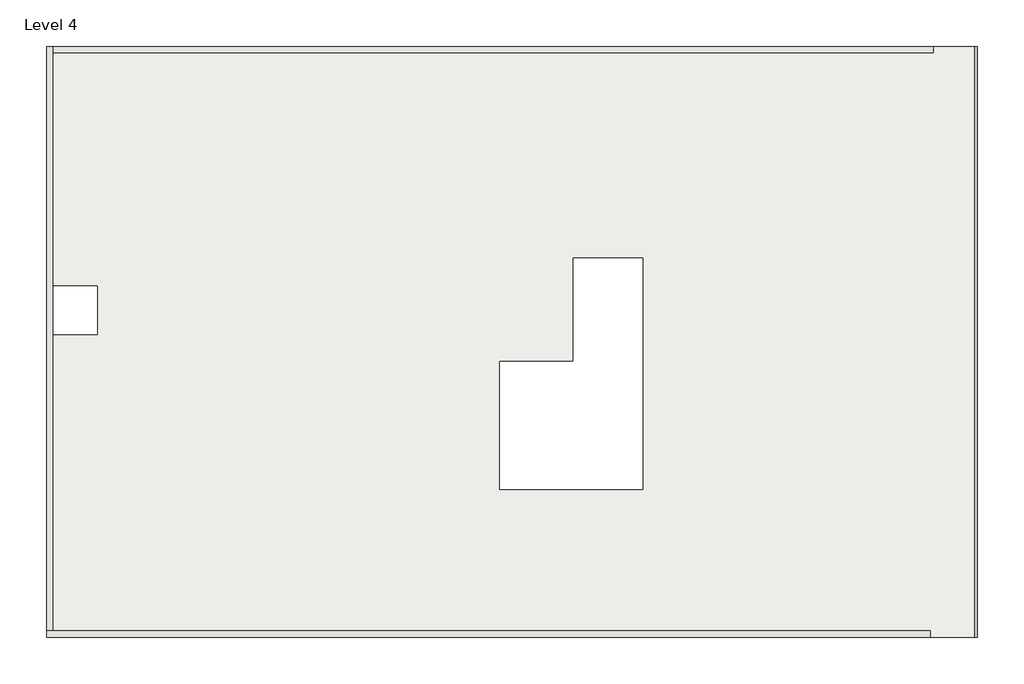
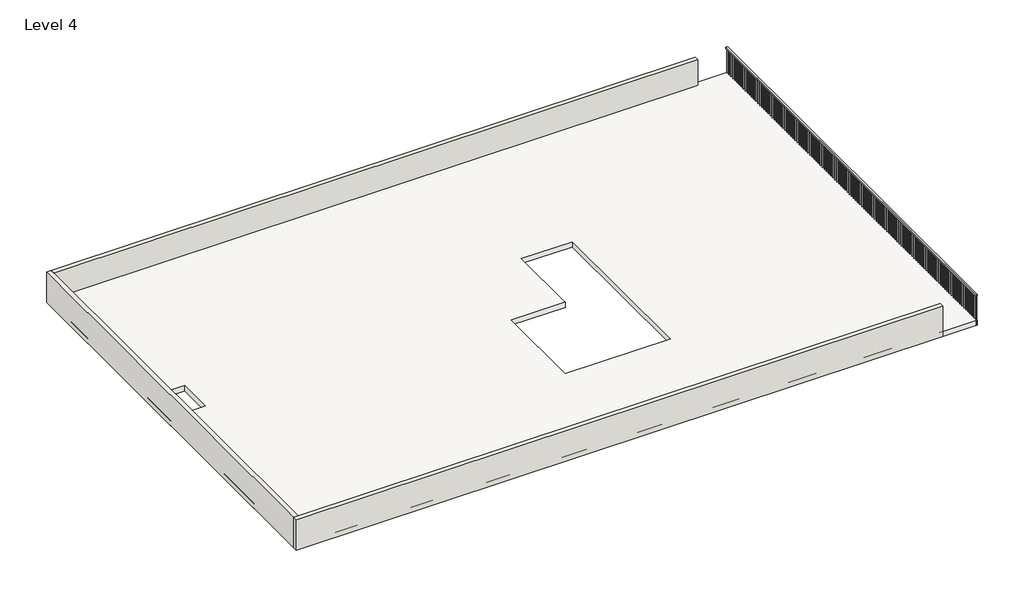
# One storey: 3 walls, 1 railing, 1 slab.
"""IFC4 building model written with IfcOpenShell, lengths in millimetres."""

from ifc_helpers import new_model, si_unit, frame, origin, place, context, project, spatial, polyline, outline, extrude, faceted_brep, element, save

model = new_model("IFC4")

# Units and contexts
model_context = context("Model", 3, world=origin())
ifc_project = project(units=[si_unit("LENGTHUNIT", "METRE", prefix="MILLI")], contexts=[model_context])

# Site, building, storey
site = spatial("IfcSite", under=ifc_project)
building = spatial("IfcBuilding", under=site)
storey = spatial("IfcBuildingStorey", under=building, Name="Level 4", Elevation=9144.0)

# Railing
placement = place(None, origin())
element("IfcRailing", 1, ObjectType="Handrail - Rectangular", at=placement, inside=storey, context=model_context, shape_type="SweptSolid", body=[
    extrude(outline(polyline([(6706.5574466, 3231.2168492), (6757.3574466, 3231.2168492), (6757.3574466, -8960.7831508), (6706.5574466, -8960.7831508), (6706.5574466, 3231.2168492)])), frame((0.0, 0.0, 10007.6), z_axis=(0.0, 0.0, 1.0), x_axis=(1.0, 0.0, 0.0)), (0.0, 0.0, 1.0), 50.8),
    extrude(outline(polyline([(6722.4324466, -8849.6581508), (6741.4824466, -8849.6581508), (6741.4824466, -8868.7081508), (6722.4324466, -8868.7081508), (6722.4324466, -8849.6581508)])), frame((0.0, 0.0, 9144.0), z_axis=(0.0, 0.0, 1.0), x_axis=(1.0, 0.0, 0.0)), (0.0, 0.0, 1.0), 863.6),
    extrude(outline(polyline([(6722.4324466, -8748.0581508), (6741.4824466, -8748.0581508), (6741.4824466, -8767.1081508), (6722.4324466, -8767.1081508), (6722.4324466, -8748.0581508)])), frame((0.0, 0.0, 9144.0), z_axis=(0.0, 0.0, 1.0), x_axis=(1.0, 0.0, 0.0)), (0.0, 0.0, 1.0), 863.6),
    extrude(outline(polyline([(6722.4324466, -8646.4581508), (6741.4824466, -8646.4581508), (6741.4824466, -8665.5081508), (6722.4324466, -8665.5081508), (6722.4324466, -8646.4581508)])), frame((0.0, 0.0, 9144.0), z_axis=(0.0, 0.0, 1.0), x_axis=(1.0, 0.0, 0.0)), (0.0, 0.0, 1.0), 863.6),
    extrude(outline(polyline([(6722.4324466, -8544.8581508), (6741.4824466, -8544.8581508), (6741.4824466, -8563.9081508), (6722.4324466, -8563.9081508), (6722.4324466, -8544.8581508)])), frame((0.0, 0.0, 9144.0), z_axis=(0.0, 0.0, 1.0), x_axis=(1.0, 0.0, 0.0)), (0.0, 0.0, 1.0), 863.6),
    extrude(outline(polyline([(6722.4324466, -8443.2581508), (6741.4824466, -8443.2581508), (6741.4824466, -8462.3081508), (6722.4324466, -8462.3081508), (6722.4324466, -8443.2581508)])), frame((0.0, 0.0, 9144.0), z_axis=(0.0, 0.0, 1.0), x_axis=(1.0, 0.0, 0.0)), (0.0, 0.0, 1.0), 863.6),
    extrude(outline(polyline([(6722.4324466, -8341.6581508), (6741.4824466, -8341.6581508), (6741.4824466, -8360.7081508), (6722.4324466, -8360.7081508), (6722.4324466, -8341.6581508)])), frame((0.0, 0.0, 9144.0), z_axis=(0.0, 0.0, 1.0), x_axis=(1.0, 0.0, 0.0)), (0.0, 0.0, 1.0), 863.6),
    extrude(outline(polyline([(6722.4324466, -8240.0581508), (6741.4824466, -8240.0581508), (6741.4824466, -8259.1081508), (6722.4324466, -8259.1081508), (6722.4324466, -8240.0581508)])), frame((0.0, 0.0, 9144.0), z_axis=(0.0, 0.0, 1.0), x_axis=(1.0, 0.0, 0.0)), (0.0, 0.0, 1.0), 863.6),
    extrude(outline(polyline([(6722.4324466, -8138.4581508), (6741.4824466, -8138.4581508), (6741.4824466, -8157.5081508), (6722.4324466, -8157.5081508), (6722.4324466, -8138.4581508)])), frame((0.0, 0.0, 9144.0), z_axis=(0.0, 0.0, 1.0), x_axis=(1.0, 0.0, 0.0)), (0.0, 0.0, 1.0), 863.6),
    extrude(outline(polyline([(6722.4324466, -8036.8581508), (6741.4824466, -8036.8581508), (6741.4824466, -8055.9081508), (6722.4324466, -8055.9081508), (6722.4324466, -8036.8581508)])), frame((0.0, 0.0, 9144.0), z_axis=(0.0, 0.0, 1.0), x_axis=(1.0, 0.0, 0.0)), (0.0, 0.0, 1.0), 863.6),
    extrude(outline(polyline([(6722.4324466, -7935.2581508), (6741.4824466, -7935.2581508), (6741.4824466, -7954.3081508), (6722.4324466, -7954.3081508), (6722.4324466, -7935.2581508)])), frame((0.0, 0.0, 9144.0), z_axis=(0.0, 0.0, 1.0), x_axis=(1.0, 0.0, 0.0)), (0.0, 0.0, 1.0), 863.6),
    extrude(outline(polyline([(6722.4324466, -7833.6581508), (6741.4824466, -7833.6581508), (6741.4824466, -7852.7081508), (6722.4324466, -7852.7081508), (6722.4324466, -7833.6581508)])), frame((0.0, 0.0, 9144.0), z_axis=(0.0, 0.0, 1.0), x_axis=(1.0, 0.0, 0.0)), (0.0, 0.0, 1.0), 863.6),
    extrude(outline(polyline([(6722.4324466, -7732.0581508), (6741.4824466, -7732.0581508), (6741.4824466, -7751.1081508), (6722.4324466, -7751.1081508), (6722.4324466, -7732.0581508)])), frame((0.0, 0.0, 9144.0), z_axis=(0.0, 0.0, 1.0), x_axis=(1.0, 0.0, 0.0)), (0.0, 0.0, 1.0), 863.6),
    extrude(outline(polyline([(6722.4324466, -7630.4581508), (6741.4824466, -7630.4581508), (6741.4824466, -7649.5081508), (6722.4324466, -7649.5081508), (6722.4324466, -7630.4581508)])), frame((0.0, 0.0, 9144.0), z_axis=(0.0, 0.0, 1.0), x_axis=(1.0, 0.0, 0.0)), (0.0, 0.0, 1.0), 863.6),
    extrude(outline(polyline([(6722.4324466, -7528.8581508), (6741.4824466, -7528.8581508), (6741.4824466, -7547.9081508), (6722.4324466, -7547.9081508), (6722.4324466, -7528.8581508)])), frame((0.0, 0.0, 9144.0), z_axis=(0.0, 0.0, 1.0), x_axis=(1.0, 0.0, 0.0)), (0.0, 0.0, 1.0), 863.6),
    extrude(outline(polyline([(6722.4324466, -7427.2581508), (6741.4824466, -7427.2581508), (6741.4824466, -7446.3081508), (6722.4324466, -7446.3081508), (6722.4324466, -7427.2581508)])), frame((0.0, 0.0, 9144.0), z_axis=(0.0, 0.0, 1.0), x_axis=(1.0, 0.0, 0.0)), (0.0, 0.0, 1.0), 863.6),
    extrude(outline(polyline([(6722.4324466, -7325.6581508), (6741.4824466, -7325.6581508), (6741.4824466, -7344.7081508), (6722.4324466, -7344.7081508), (6722.4324466, -7325.6581508)])), frame((0.0, 0.0, 9144.0), z_axis=(0.0, 0.0, 1.0), x_axis=(1.0, 0.0, 0.0)), (0.0, 0.0, 1.0), 863.6),
    extrude(outline(polyline([(6722.4324466, -7224.0581508), (6741.4824466, -7224.0581508), (6741.4824466, -7243.1081508), (6722.4324466, -7243.1081508), (6722.4324466, -7224.0581508)])), frame((0.0, 0.0, 9144.0), z_axis=(0.0, 0.0, 1.0), x_axis=(1.0, 0.0, 0.0)), (0.0, 0.0, 1.0), 863.6),
    extrude(outline(polyline([(6722.4324466, -7122.4581508), (6741.4824466, -7122.4581508), (6741.4824466, -7141.5081508), (6722.4324466, -7141.5081508), (6722.4324466, -7122.4581508)])), frame((0.0, 0.0, 9144.0), z_axis=(0.0, 0.0, 1.0), x_axis=(1.0, 0.0, 0.0)), (0.0, 0.0, 1.0), 863.6),
    extrude(outline(polyline([(6722.4324466, -7020.8581508), (6741.4824466, -7020.8581508), (6741.4824466, -7039.9081508), (6722.4324466, -7039.9081508), (6722.4324466, -7020.8581508)])), frame((0.0, 0.0, 9144.0), z_axis=(0.0, 0.0, 1.0), x_axis=(1.0, 0.0, 0.0)), (0.0, 0.0, 1.0), 863.6),
    extrude(outline(polyline([(6722.4324466, -6919.2581508), (6741.4824466, -6919.2581508), (6741.4824466, -6938.3081508), (6722.4324466, -6938.3081508), (6722.4324466, -6919.2581508)])), frame((0.0, 0.0, 9144.0), z_axis=(0.0, 0.0, 1.0), x_axis=(1.0, 0.0, 0.0)), (0.0, 0.0, 1.0), 863.6),
    extrude(outline(polyline([(6722.4324466, -6817.6581508), (6741.4824466, -6817.6581508), (6741.4824466, -6836.7081508), (6722.4324466, -6836.7081508), (6722.4324466, -6817.6581508)])), frame((0.0, 0.0, 9144.0), z_axis=(0.0, 0.0, 1.0), x_axis=(1.0, 0.0, 0.0)), (0.0, 0.0, 1.0), 863.6),
    extrude(outline(polyline([(6722.4324466, -6716.0581508), (6741.4824466, -6716.0581508), (6741.4824466, -6735.1081508), (6722.4324466, -6735.1081508), (6722.4324466, -6716.0581508)])), frame((0.0, 0.0, 9144.0), z_axis=(0.0, 0.0, 1.0), x_axis=(1.0, 0.0, 0.0)), (0.0, 0.0, 1.0), 863.6),
    extrude(outline(polyline([(6722.4324466, -6614.4581508), (6741.4824466, -6614.4581508), (6741.4824466, -6633.5081508), (6722.4324466, -6633.5081508), (6722.4324466, -6614.4581508)])), frame((0.0, 0.0, 9144.0), z_axis=(0.0, 0.0, 1.0), x_axis=(1.0, 0.0, 0.0)), (0.0, 0.0, 1.0), 863.6),
    extrude(outline(polyline([(6722.4324466, -6512.8581508), (6741.4824466, -6512.8581508), (6741.4824466, -6531.9081508), (6722.4324466, -6531.9081508), (6722.4324466, -6512.8581508)])), frame((0.0, 0.0, 9144.0), z_axis=(0.0, 0.0, 1.0), x_axis=(1.0, 0.0, 0.0)), (0.0, 0.0, 1.0), 863.6),
    extrude(outline(polyline([(6722.4324466, -6411.2581508), (6741.4824466, -6411.2581508), (6741.4824466, -6430.3081508), (6722.4324466, -6430.3081508), (6722.4324466, -6411.2581508)])), frame((0.0, 0.0, 9144.0), z_axis=(0.0, 0.0, 1.0), x_axis=(1.0, 0.0, 0.0)), (0.0, 0.0, 1.0), 863.6),
    extrude(outline(polyline([(6722.4324466, -6309.6581508), (6741.4824466, -6309.6581508), (6741.4824466, -6328.7081508), (6722.4324466, -6328.7081508), (6722.4324466, -6309.6581508)])), frame((0.0, 0.0, 9144.0), z_axis=(0.0, 0.0, 1.0), x_axis=(1.0, 0.0, 0.0)), (0.0, 0.0, 1.0), 863.6),
    extrude(outline(polyline([(6722.4324466, -6208.0581508), (6741.4824466, -6208.0581508), (6741.4824466, -6227.1081508), (6722.4324466, -6227.1081508), (6722.4324466, -6208.0581508)])), frame((0.0, 0.0, 9144.0), z_axis=(0.0, 0.0, 1.0), x_axis=(1.0, 0.0, 0.0)), (0.0, 0.0, 1.0), 863.6),
    extrude(outline(polyline([(6722.4324466, -6106.4581508), (6741.4824466, -6106.4581508), (6741.4824466, -6125.5081508), (6722.4324466, -6125.5081508), (6722.4324466, -6106.4581508)])), frame((0.0, 0.0, 9144.0), z_axis=(0.0, 0.0, 1.0), x_axis=(1.0, 0.0, 0.0)), (0.0, 0.0, 1.0), 863.6),
    extrude(outline(polyline([(6722.4324466, -6004.8581508), (6741.4824466, -6004.8581508), (6741.4824466, -6023.9081508), (6722.4324466, -6023.9081508), (6722.4324466, -6004.8581508)])), frame((0.0, 0.0, 9144.0), z_axis=(0.0, 0.0, 1.0), x_axis=(1.0, 0.0, 0.0)), (0.0, 0.0, 1.0), 863.6),
    extrude(outline(polyline([(6722.4324466, -5903.2581508), (6741.4824466, -5903.2581508), (6741.4824466, -5922.3081508), (6722.4324466, -5922.3081508), (6722.4324466, -5903.2581508)])), frame((0.0, 0.0, 9144.0), z_axis=(0.0, 0.0, 1.0), x_axis=(1.0, 0.0, 0.0)), (0.0, 0.0, 1.0), 863.6),
    extrude(outline(polyline([(6722.4324466, -5801.6581508), (6741.4824466, -5801.6581508), (6741.4824466, -5820.7081508), (6722.4324466, -5820.7081508), (6722.4324466, -5801.6581508)])), frame((0.0, 0.0, 9144.0), z_axis=(0.0, 0.0, 1.0), x_axis=(1.0, 0.0, 0.0)), (0.0, 0.0, 1.0), 863.6),
    extrude(outline(polyline([(6722.4324466, -5700.0581508), (6741.4824466, -5700.0581508), (6741.4824466, -5719.1081508), (6722.4324466, -5719.1081508), (6722.4324466, -5700.0581508)])), frame((0.0, 0.0, 9144.0), z_axis=(0.0, 0.0, 1.0), x_axis=(1.0, 0.0, 0.0)), (0.0, 0.0, 1.0), 863.6),
    extrude(outline(polyline([(6722.4324466, -5598.4581508), (6741.4824466, -5598.4581508), (6741.4824466, -5617.5081508), (6722.4324466, -5617.5081508), (6722.4324466, -5598.4581508)])), frame((0.0, 0.0, 9144.0), z_axis=(0.0, 0.0, 1.0), x_axis=(1.0, 0.0, 0.0)), (0.0, 0.0, 1.0), 863.6),
    extrude(outline(polyline([(6722.4324466, -5496.8581508), (6741.4824466, -5496.8581508), (6741.4824466, -5515.9081508), (6722.4324466, -5515.9081508), (6722.4324466, -5496.8581508)])), frame((0.0, 0.0, 9144.0), z_axis=(0.0, 0.0, 1.0), x_axis=(1.0, 0.0, 0.0)), (0.0, 0.0, 1.0), 863.6),
    extrude(outline(polyline([(6722.4324466, -5395.2581508), (6741.4824466, -5395.2581508), (6741.4824466, -5414.3081508), (6722.4324466, -5414.3081508), (6722.4324466, -5395.2581508)])), frame((0.0, 0.0, 9144.0), z_axis=(0.0, 0.0, 1.0), x_axis=(1.0, 0.0, 0.0)), (0.0, 0.0, 1.0), 863.6),
    extrude(outline(polyline([(6722.4324466, -5293.6581508), (6741.4824466, -5293.6581508), (6741.4824466, -5312.7081508), (6722.4324466, -5312.7081508), (6722.4324466, -5293.6581508)])), frame((0.0, 0.0, 9144.0), z_axis=(0.0, 0.0, 1.0), x_axis=(1.0, 0.0, 0.0)), (0.0, 0.0, 1.0), 863.6),
    extrude(outline(polyline([(6722.4324466, -5192.0581508), (6741.4824466, -5192.0581508), (6741.4824466, -5211.1081508), (6722.4324466, -5211.1081508), (6722.4324466, -5192.0581508)])), frame((0.0, 0.0, 9144.0), z_axis=(0.0, 0.0, 1.0), x_axis=(1.0, 0.0, 0.0)), (0.0, 0.0, 1.0), 863.6),
    extrude(outline(polyline([(6722.4324466, -5090.4581508), (6741.4824466, -5090.4581508), (6741.4824466, -5109.5081508), (6722.4324466, -5109.5081508), (6722.4324466, -5090.4581508)])), frame((0.0, 0.0, 9144.0), z_axis=(0.0, 0.0, 1.0), x_axis=(1.0, 0.0, 0.0)), (0.0, 0.0, 1.0), 863.6),
    extrude(outline(polyline([(6722.4324466, -4988.8581508), (6741.4824466, -4988.8581508), (6741.4824466, -5007.9081508), (6722.4324466, -5007.9081508), (6722.4324466, -4988.8581508)])), frame((0.0, 0.0, 9144.0), z_axis=(0.0, 0.0, 1.0), x_axis=(1.0, 0.0, 0.0)), (0.0, 0.0, 1.0), 863.6),
    extrude(outline(polyline([(6722.4324466, -4887.2581508), (6741.4824466, -4887.2581508), (6741.4824466, -4906.3081508), (6722.4324466, -4906.3081508), (6722.4324466, -4887.2581508)])), frame((0.0, 0.0, 9144.0), z_axis=(0.0, 0.0, 1.0), x_axis=(1.0, 0.0, 0.0)), (0.0, 0.0, 1.0), 863.6),
    extrude(outline(polyline([(6722.4324466, -4785.6581508), (6741.4824466, -4785.6581508), (6741.4824466, -4804.7081508), (6722.4324466, -4804.7081508), (6722.4324466, -4785.6581508)])), frame((0.0, 0.0, 9144.0), z_axis=(0.0, 0.0, 1.0), x_axis=(1.0, 0.0, 0.0)), (0.0, 0.0, 1.0), 863.6),
    extrude(outline(polyline([(6722.4324466, -4684.0581508), (6741.4824466, -4684.0581508), (6741.4824466, -4703.1081508), (6722.4324466, -4703.1081508), (6722.4324466, -4684.0581508)])), frame((0.0, 0.0, 9144.0), z_axis=(0.0, 0.0, 1.0), x_axis=(1.0, 0.0, 0.0)), (0.0, 0.0, 1.0), 863.6),
    extrude(outline(polyline([(6722.4324466, -4582.4581508), (6741.4824466, -4582.4581508), (6741.4824466, -4601.5081508), (6722.4324466, -4601.5081508), (6722.4324466, -4582.4581508)])), frame((0.0, 0.0, 9144.0), z_axis=(0.0, 0.0, 1.0), x_axis=(1.0, 0.0, 0.0)), (0.0, 0.0, 1.0), 863.6),
    extrude(outline(polyline([(6722.4324466, -4480.8581508), (6741.4824466, -4480.8581508), (6741.4824466, -4499.9081508), (6722.4324466, -4499.9081508), (6722.4324466, -4480.8581508)])), frame((0.0, 0.0, 9144.0), z_axis=(0.0, 0.0, 1.0), x_axis=(1.0, 0.0, 0.0)), (0.0, 0.0, 1.0), 863.6),
    extrude(outline(polyline([(6722.4324466, -4379.2581508), (6741.4824466, -4379.2581508), (6741.4824466, -4398.3081508), (6722.4324466, -4398.3081508), (6722.4324466, -4379.2581508)])), frame((0.0, 0.0, 9144.0), z_axis=(0.0, 0.0, 1.0), x_axis=(1.0, 0.0, 0.0)), (0.0, 0.0, 1.0), 863.6),
    extrude(outline(polyline([(6722.4324466, -4277.6581508), (6741.4824466, -4277.6581508), (6741.4824466, -4296.7081508), (6722.4324466, -4296.7081508), (6722.4324466, -4277.6581508)])), frame((0.0, 0.0, 9144.0), z_axis=(0.0, 0.0, 1.0), x_axis=(1.0, 0.0, 0.0)), (0.0, 0.0, 1.0), 863.6),
    extrude(outline(polyline([(6722.4324466, -4176.0581508), (6741.4824466, -4176.0581508), (6741.4824466, -4195.1081508), (6722.4324466, -4195.1081508), (6722.4324466, -4176.0581508)])), frame((0.0, 0.0, 9144.0), z_axis=(0.0, 0.0, 1.0), x_axis=(1.0, 0.0, 0.0)), (0.0, 0.0, 1.0), 863.6),
    extrude(outline(polyline([(6722.4324466, -4074.4581508), (6741.4824466, -4074.4581508), (6741.4824466, -4093.5081508), (6722.4324466, -4093.5081508), (6722.4324466, -4074.4581508)])), frame((0.0, 0.0, 9144.0), z_axis=(0.0, 0.0, 1.0), x_axis=(1.0, 0.0, 0.0)), (0.0, 0.0, 1.0), 863.6),
    extrude(outline(polyline([(6722.4324466, -3972.8581508), (6741.4824466, -3972.8581508), (6741.4824466, -3991.9081508), (6722.4324466, -3991.9081508), (6722.4324466, -3972.8581508)])), frame((0.0, 0.0, 9144.0), z_axis=(0.0, 0.0, 1.0), x_axis=(1.0, 0.0, 0.0)), (0.0, 0.0, 1.0), 863.6),
    extrude(outline(polyline([(6722.4324466, -3871.2581508), (6741.4824466, -3871.2581508), (6741.4824466, -3890.3081508), (6722.4324466, -3890.3081508), (6722.4324466, -3871.2581508)])), frame((0.0, 0.0, 9144.0), z_axis=(0.0, 0.0, 1.0), x_axis=(1.0, 0.0, 0.0)), (0.0, 0.0, 1.0), 863.6),
    extrude(outline(polyline([(6722.4324466, -3769.6581508), (6741.4824466, -3769.6581508), (6741.4824466, -3788.7081508), (6722.4324466, -3788.7081508), (6722.4324466, -3769.6581508)])), frame((0.0, 0.0, 9144.0), z_axis=(0.0, 0.0, 1.0), x_axis=(1.0, 0.0, 0.0)), (0.0, 0.0, 1.0), 863.6),
    extrude(outline(polyline([(6722.4324466, -3668.0581508), (6741.4824466, -3668.0581508), (6741.4824466, -3687.1081508), (6722.4324466, -3687.1081508), (6722.4324466, -3668.0581508)])), frame((0.0, 0.0, 9144.0), z_axis=(0.0, 0.0, 1.0), x_axis=(1.0, 0.0, 0.0)), (0.0, 0.0, 1.0), 863.6),
    extrude(outline(polyline([(6722.4324466, -3566.4581508), (6741.4824466, -3566.4581508), (6741.4824466, -3585.5081508), (6722.4324466, -3585.5081508), (6722.4324466, -3566.4581508)])), frame((0.0, 0.0, 9144.0), z_axis=(0.0, 0.0, 1.0), x_axis=(1.0, 0.0, 0.0)), (0.0, 0.0, 1.0), 863.6),
    extrude(outline(polyline([(6722.4324466, -3464.8581508), (6741.4824466, -3464.8581508), (6741.4824466, -3483.9081508), (6722.4324466, -3483.9081508), (6722.4324466, -3464.8581508)])), frame((0.0, 0.0, 9144.0), z_axis=(0.0, 0.0, 1.0), x_axis=(1.0, 0.0, 0.0)), (0.0, 0.0, 1.0), 863.6),
    extrude(outline(polyline([(6722.4324466, -3363.2581508), (6741.4824466, -3363.2581508), (6741.4824466, -3382.3081508), (6722.4324466, -3382.3081508), (6722.4324466, -3363.2581508)])), frame((0.0, 0.0, 9144.0), z_axis=(0.0, 0.0, 1.0), x_axis=(1.0, 0.0, 0.0)), (0.0, 0.0, 1.0), 863.6),
    extrude(outline(polyline([(6722.4324466, -3261.6581508), (6741.4824466, -3261.6581508), (6741.4824466, -3280.7081508), (6722.4324466, -3280.7081508), (6722.4324466, -3261.6581508)])), frame((0.0, 0.0, 9144.0), z_axis=(0.0, 0.0, 1.0), x_axis=(1.0, 0.0, 0.0)), (0.0, 0.0, 1.0), 863.6),
    extrude(outline(polyline([(6722.4324466, -3160.0581508), (6741.4824466, -3160.0581508), (6741.4824466, -3179.1081508), (6722.4324466, -3179.1081508), (6722.4324466, -3160.0581508)])), frame((0.0, 0.0, 9144.0), z_axis=(0.0, 0.0, 1.0), x_axis=(1.0, 0.0, 0.0)), (0.0, 0.0, 1.0), 863.6),
    extrude(outline(polyline([(6722.4324466, -3058.4581508), (6741.4824466, -3058.4581508), (6741.4824466, -3077.5081508), (6722.4324466, -3077.5081508), (6722.4324466, -3058.4581508)])), frame((0.0, 0.0, 9144.0), z_axis=(0.0, 0.0, 1.0), x_axis=(1.0, 0.0, 0.0)), (0.0, 0.0, 1.0), 863.6),
    extrude(outline(polyline([(6722.4324466, -2956.8581508), (6741.4824466, -2956.8581508), (6741.4824466, -2975.9081508), (6722.4324466, -2975.9081508), (6722.4324466, -2956.8581508)])), frame((0.0, 0.0, 9144.0), z_axis=(0.0, 0.0, 1.0), x_axis=(1.0, 0.0, 0.0)), (0.0, 0.0, 1.0), 863.6),
    extrude(outline(polyline([(6722.4324466, -2855.2581508), (6741.4824466, -2855.2581508), (6741.4824466, -2874.3081508), (6722.4324466, -2874.3081508), (6722.4324466, -2855.2581508)])), frame((0.0, 0.0, 9144.0), z_axis=(0.0, 0.0, 1.0), x_axis=(1.0, 0.0, 0.0)), (0.0, 0.0, 1.0), 863.6),
    extrude(outline(polyline([(6722.4324466, -2753.6581508), (6741.4824466, -2753.6581508), (6741.4824466, -2772.7081508), (6722.4324466, -2772.7081508), (6722.4324466, -2753.6581508)])), frame((0.0, 0.0, 9144.0), z_axis=(0.0, 0.0, 1.0), x_axis=(1.0, 0.0, 0.0)), (0.0, 0.0, 1.0), 863.6),
    extrude(outline(polyline([(6722.4324466, -2652.0581508), (6741.4824466, -2652.0581508), (6741.4824466, -2671.1081508), (6722.4324466, -2671.1081508), (6722.4324466, -2652.0581508)])), frame((0.0, 0.0, 9144.0), z_axis=(0.0, 0.0, 1.0), x_axis=(1.0, 0.0, 0.0)), (0.0, 0.0, 1.0), 863.6),
    extrude(outline(polyline([(6722.4324466, -2550.4581508), (6741.4824466, -2550.4581508), (6741.4824466, -2569.5081508), (6722.4324466, -2569.5081508), (6722.4324466, -2550.4581508)])), frame((0.0, 0.0, 9144.0), z_axis=(0.0, 0.0, 1.0), x_axis=(1.0, 0.0, 0.0)), (0.0, 0.0, 1.0), 863.6),
    extrude(outline(polyline([(6722.4324466, -2448.8581508), (6741.4824466, -2448.8581508), (6741.4824466, -2467.9081508), (6722.4324466, -2467.9081508), (6722.4324466, -2448.8581508)])), frame((0.0, 0.0, 9144.0), z_axis=(0.0, 0.0, 1.0), x_axis=(1.0, 0.0, 0.0)), (0.0, 0.0, 1.0), 863.6),
    extrude(outline(polyline([(6722.4324466, -2347.2581508), (6741.4824466, -2347.2581508), (6741.4824466, -2366.3081508), (6722.4324466, -2366.3081508), (6722.4324466, -2347.2581508)])), frame((0.0, 0.0, 9144.0), z_axis=(0.0, 0.0, 1.0), x_axis=(1.0, 0.0, 0.0)), (0.0, 0.0, 1.0), 863.6),
    extrude(outline(polyline([(6722.4324466, -2245.6581508), (6741.4824466, -2245.6581508), (6741.4824466, -2264.7081508), (6722.4324466, -2264.7081508), (6722.4324466, -2245.6581508)])), frame((0.0, 0.0, 9144.0), z_axis=(0.0, 0.0, 1.0), x_axis=(1.0, 0.0, 0.0)), (0.0, 0.0, 1.0), 863.6),
    extrude(outline(polyline([(6722.4324466, -2144.0581508), (6741.4824466, -2144.0581508), (6741.4824466, -2163.1081508), (6722.4324466, -2163.1081508), (6722.4324466, -2144.0581508)])), frame((0.0, 0.0, 9144.0), z_axis=(0.0, 0.0, 1.0), x_axis=(1.0, 0.0, 0.0)), (0.0, 0.0, 1.0), 863.6),
    extrude(outline(polyline([(6722.4324466, -2042.4581508), (6741.4824466, -2042.4581508), (6741.4824466, -2061.5081508), (6722.4324466, -2061.5081508), (6722.4324466, -2042.4581508)])), frame((0.0, 0.0, 9144.0), z_axis=(0.0, 0.0, 1.0), x_axis=(1.0, 0.0, 0.0)), (0.0, 0.0, 1.0), 863.6),
    extrude(outline(polyline([(6722.4324466, -1940.8581508), (6741.4824466, -1940.8581508), (6741.4824466, -1959.9081508), (6722.4324466, -1959.9081508), (6722.4324466, -1940.8581508)])), frame((0.0, 0.0, 9144.0), z_axis=(0.0, 0.0, 1.0), x_axis=(1.0, 0.0, 0.0)), (0.0, 0.0, 1.0), 863.6),
    extrude(outline(polyline([(6722.4324466, -1839.2581508), (6741.4824466, -1839.2581508), (6741.4824466, -1858.3081508), (6722.4324466, -1858.3081508), (6722.4324466, -1839.2581508)])), frame((0.0, 0.0, 9144.0), z_axis=(0.0, 0.0, 1.0), x_axis=(1.0, 0.0, 0.0)), (0.0, 0.0, 1.0), 863.6),
    extrude(outline(polyline([(6722.4324466, -1737.6581508), (6741.4824466, -1737.6581508), (6741.4824466, -1756.7081508), (6722.4324466, -1756.7081508), (6722.4324466, -1737.6581508)])), frame((0.0, 0.0, 9144.0), z_axis=(0.0, 0.0, 1.0), x_axis=(1.0, 0.0, 0.0)), (0.0, 0.0, 1.0), 863.6),
    extrude(outline(polyline([(6722.4324466, -1636.0581508), (6741.4824466, -1636.0581508), (6741.4824466, -1655.1081508), (6722.4324466, -1655.1081508), (6722.4324466, -1636.0581508)])), frame((0.0, 0.0, 9144.0), z_axis=(0.0, 0.0, 1.0), x_axis=(1.0, 0.0, 0.0)), (0.0, 0.0, 1.0), 863.6),
    extrude(outline(polyline([(6722.4324466, -1534.4581508), (6741.4824466, -1534.4581508), (6741.4824466, -1553.5081508), (6722.4324466, -1553.5081508), (6722.4324466, -1534.4581508)])), frame((0.0, 0.0, 9144.0), z_axis=(0.0, 0.0, 1.0), x_axis=(1.0, 0.0, 0.0)), (0.0, 0.0, 1.0), 863.6),
    extrude(outline(polyline([(6722.4324466, -1432.8581508), (6741.4824466, -1432.8581508), (6741.4824466, -1451.9081508), (6722.4324466, -1451.9081508), (6722.4324466, -1432.8581508)])), frame((0.0, 0.0, 9144.0), z_axis=(0.0, 0.0, 1.0), x_axis=(1.0, 0.0, 0.0)), (0.0, 0.0, 1.0), 863.6),
    extrude(outline(polyline([(6722.4324466, -1331.2581508), (6741.4824466, -1331.2581508), (6741.4824466, -1350.3081508), (6722.4324466, -1350.3081508), (6722.4324466, -1331.2581508)])), frame((0.0, 0.0, 9144.0), z_axis=(0.0, 0.0, 1.0), x_axis=(1.0, 0.0, 0.0)), (0.0, 0.0, 1.0), 863.6),
    extrude(outline(polyline([(6722.4324466, -1229.6581508), (6741.4824466, -1229.6581508), (6741.4824466, -1248.7081508), (6722.4324466, -1248.7081508), (6722.4324466, -1229.6581508)])), frame((0.0, 0.0, 9144.0), z_axis=(0.0, 0.0, 1.0), x_axis=(1.0, 0.0, 0.0)), (0.0, 0.0, 1.0), 863.6),
    extrude(outline(polyline([(6722.4324466, -1128.0581508), (6741.4824466, -1128.0581508), (6741.4824466, -1147.1081508), (6722.4324466, -1147.1081508), (6722.4324466, -1128.0581508)])), frame((0.0, 0.0, 9144.0), z_axis=(0.0, 0.0, 1.0), x_axis=(1.0, 0.0, 0.0)), (0.0, 0.0, 1.0), 863.6),
    extrude(outline(polyline([(6722.4324466, -1026.4581508), (6741.4824466, -1026.4581508), (6741.4824466, -1045.5081508), (6722.4324466, -1045.5081508), (6722.4324466, -1026.4581508)])), frame((0.0, 0.0, 9144.0), z_axis=(0.0, 0.0, 1.0), x_axis=(1.0, 0.0, 0.0)), (0.0, 0.0, 1.0), 863.6),
    extrude(outline(polyline([(6722.4324466, -924.8581508), (6741.4824466, -924.8581508), (6741.4824466, -943.9081508), (6722.4324466, -943.9081508), (6722.4324466, -924.8581508)])), frame((0.0, 0.0, 9144.0), z_axis=(0.0, 0.0, 1.0), x_axis=(1.0, 0.0, 0.0)), (0.0, 0.0, 1.0), 863.6),
    extrude(outline(polyline([(6722.4324466, -823.2581508), (6741.4824466, -823.2581508), (6741.4824466, -842.3081508), (6722.4324466, -842.3081508), (6722.4324466, -823.2581508)])), frame((0.0, 0.0, 9144.0), z_axis=(0.0, 0.0, 1.0), x_axis=(1.0, 0.0, 0.0)), (0.0, 0.0, 1.0), 863.6),
    extrude(outline(polyline([(6722.4324466, -721.6581508), (6741.4824466, -721.6581508), (6741.4824466, -740.7081508), (6722.4324466, -740.7081508), (6722.4324466, -721.6581508)])), frame((0.0, 0.0, 9144.0), z_axis=(0.0, 0.0, 1.0), x_axis=(1.0, 0.0, 0.0)), (0.0, 0.0, 1.0), 863.6),
    extrude(outline(polyline([(6722.4324466, -620.0581508), (6741.4824466, -620.0581508), (6741.4824466, -639.1081508), (6722.4324466, -639.1081508), (6722.4324466, -620.0581508)])), frame((0.0, 0.0, 9144.0), z_axis=(0.0, 0.0, 1.0), x_axis=(1.0, 0.0, 0.0)), (0.0, 0.0, 1.0), 863.6),
    extrude(outline(polyline([(6722.4324466, -518.4581508), (6741.4824466, -518.4581508), (6741.4824466, -537.5081508), (6722.4324466, -537.5081508), (6722.4324466, -518.4581508)])), frame((0.0, 0.0, 9144.0), z_axis=(0.0, 0.0, 1.0), x_axis=(1.0, 0.0, 0.0)), (0.0, 0.0, 1.0), 863.6),
    extrude(outline(polyline([(6722.4324466, -416.8581508), (6741.4824466, -416.8581508), (6741.4824466, -435.9081508), (6722.4324466, -435.9081508), (6722.4324466, -416.8581508)])), frame((0.0, 0.0, 9144.0), z_axis=(0.0, 0.0, 1.0), x_axis=(1.0, 0.0, 0.0)), (0.0, 0.0, 1.0), 863.6),
    extrude(outline(polyline([(6722.4324466, -315.2581508), (6741.4824466, -315.2581508), (6741.4824466, -334.3081508), (6722.4324466, -334.3081508), (6722.4324466, -315.2581508)])), frame((0.0, 0.0, 9144.0), z_axis=(0.0, 0.0, 1.0), x_axis=(1.0, 0.0, 0.0)), (0.0, 0.0, 1.0), 863.6),
    extrude(outline(polyline([(6722.4324466, -213.6581508), (6741.4824466, -213.6581508), (6741.4824466, -232.7081508), (6722.4324466, -232.7081508), (6722.4324466, -213.6581508)])), frame((0.0, 0.0, 9144.0), z_axis=(0.0, 0.0, 1.0), x_axis=(1.0, 0.0, 0.0)), (0.0, 0.0, 1.0), 863.6),
    extrude(outline(polyline([(6722.4324466, -112.0581508), (6741.4824466, -112.0581508), (6741.4824466, -131.1081508), (6722.4324466, -131.1081508), (6722.4324466, -112.0581508)])), frame((0.0, 0.0, 9144.0), z_axis=(0.0, 0.0, 1.0), x_axis=(1.0, 0.0, 0.0)), (0.0, 0.0, 1.0), 863.6),
    extrude(outline(polyline([(6722.4324466, -10.4581508), (6741.4824466, -10.4581508), (6741.4824466, -29.5081508), (6722.4324466, -29.5081508), (6722.4324466, -10.4581508)])), frame((0.0, 0.0, 9144.0), z_axis=(0.0, 0.0, 1.0), x_axis=(1.0, 0.0, 0.0)), (0.0, 0.0, 1.0), 863.6),
    extrude(outline(polyline([(6722.4324466, 91.1418492), (6741.4824466, 91.1418492), (6741.4824466, 72.0918492), (6722.4324466, 72.0918492), (6722.4324466, 91.1418492)])), frame((0.0, 0.0, 9144.0), z_axis=(0.0, 0.0, 1.0), x_axis=(1.0, 0.0, 0.0)), (0.0, 0.0, 1.0), 863.6),
    extrude(outline(polyline([(6722.4324466, 192.7418492), (6741.4824466, 192.7418492), (6741.4824466, 173.6918492), (6722.4324466, 173.6918492), (6722.4324466, 192.7418492)])), frame((0.0, 0.0, 9144.0), z_axis=(0.0, 0.0, 1.0), x_axis=(1.0, 0.0, 0.0)), (0.0, 0.0, 1.0), 863.6),
    extrude(outline(polyline([(6722.4324466, 294.3418492), (6741.4824466, 294.3418492), (6741.4824466, 275.2918492), (6722.4324466, 275.2918492), (6722.4324466, 294.3418492)])), frame((0.0, 0.0, 9144.0), z_axis=(0.0, 0.0, 1.0), x_axis=(1.0, 0.0, 0.0)), (0.0, 0.0, 1.0), 863.6),
    extrude(outline(polyline([(6722.4324466, 395.9418492), (6741.4824466, 395.9418492), (6741.4824466, 376.8918492), (6722.4324466, 376.8918492), (6722.4324466, 395.9418492)])), frame((0.0, 0.0, 9144.0), z_axis=(0.0, 0.0, 1.0), x_axis=(1.0, 0.0, 0.0)), (0.0, 0.0, 1.0), 863.6),
    extrude(outline(polyline([(6722.4324466, 497.5418492), (6741.4824466, 497.5418492), (6741.4824466, 478.4918492), (6722.4324466, 478.4918492), (6722.4324466, 497.5418492)])), frame((0.0, 0.0, 9144.0), z_axis=(0.0, 0.0, 1.0), x_axis=(1.0, 0.0, 0.0)), (0.0, 0.0, 1.0), 863.6),
    extrude(outline(polyline([(6722.4324466, 599.1418492), (6741.4824466, 599.1418492), (6741.4824466, 580.0918492), (6722.4324466, 580.0918492), (6722.4324466, 599.1418492)])), frame((0.0, 0.0, 9144.0), z_axis=(0.0, 0.0, 1.0), x_axis=(1.0, 0.0, 0.0)), (0.0, 0.0, 1.0), 863.6),
    extrude(outline(polyline([(6722.4324466, 700.7418492), (6741.4824466, 700.7418492), (6741.4824466, 681.6918492), (6722.4324466, 681.6918492), (6722.4324466, 700.7418492)])), frame((0.0, 0.0, 9144.0), z_axis=(0.0, 0.0, 1.0), x_axis=(1.0, 0.0, 0.0)), (0.0, 0.0, 1.0), 863.6),
    extrude(outline(polyline([(6722.4324466, 802.3418492), (6741.4824466, 802.3418492), (6741.4824466, 783.2918492), (6722.4324466, 783.2918492), (6722.4324466, 802.3418492)])), frame((0.0, 0.0, 9144.0), z_axis=(0.0, 0.0, 1.0), x_axis=(1.0, 0.0, 0.0)), (0.0, 0.0, 1.0), 863.6),
    extrude(outline(polyline([(6722.4324466, 903.9418492), (6741.4824466, 903.9418492), (6741.4824466, 884.8918492), (6722.4324466, 884.8918492), (6722.4324466, 903.9418492)])), frame((0.0, 0.0, 9144.0), z_axis=(0.0, 0.0, 1.0), x_axis=(1.0, 0.0, 0.0)), (0.0, 0.0, 1.0), 863.6),
    extrude(outline(polyline([(6722.4324466, 1005.5418492), (6741.4824466, 1005.5418492), (6741.4824466, 986.4918492), (6722.4324466, 986.4918492), (6722.4324466, 1005.5418492)])), frame((0.0, 0.0, 9144.0), z_axis=(0.0, 0.0, 1.0), x_axis=(1.0, 0.0, 0.0)), (0.0, 0.0, 1.0), 863.6),
    extrude(outline(polyline([(6722.4324466, 1107.1418492), (6741.4824466, 1107.1418492), (6741.4824466, 1088.0918492), (6722.4324466, 1088.0918492), (6722.4324466, 1107.1418492)])), frame((0.0, 0.0, 9144.0), z_axis=(0.0, 0.0, 1.0), x_axis=(1.0, 0.0, 0.0)), (0.0, 0.0, 1.0), 863.6),
    extrude(outline(polyline([(6722.4324466, 1208.7418492), (6741.4824466, 1208.7418492), (6741.4824466, 1189.6918492), (6722.4324466, 1189.6918492), (6722.4324466, 1208.7418492)])), frame((0.0, 0.0, 9144.0), z_axis=(0.0, 0.0, 1.0), x_axis=(1.0, 0.0, 0.0)), (0.0, 0.0, 1.0), 863.6),
    extrude(outline(polyline([(6722.4324466, 1310.3418492), (6741.4824466, 1310.3418492), (6741.4824466, 1291.2918492), (6722.4324466, 1291.2918492), (6722.4324466, 1310.3418492)])), frame((0.0, 0.0, 9144.0), z_axis=(0.0, 0.0, 1.0), x_axis=(1.0, 0.0, 0.0)), (0.0, 0.0, 1.0), 863.6),
    extrude(outline(polyline([(6722.4324466, 1411.9418492), (6741.4824466, 1411.9418492), (6741.4824466, 1392.8918492), (6722.4324466, 1392.8918492), (6722.4324466, 1411.9418492)])), frame((0.0, 0.0, 9144.0), z_axis=(0.0, 0.0, 1.0), x_axis=(1.0, 0.0, 0.0)), (0.0, 0.0, 1.0), 863.6),
    extrude(outline(polyline([(6722.4324466, 1513.5418492), (6741.4824466, 1513.5418492), (6741.4824466, 1494.4918492), (6722.4324466, 1494.4918492), (6722.4324466, 1513.5418492)])), frame((0.0, 0.0, 9144.0), z_axis=(0.0, 0.0, 1.0), x_axis=(1.0, 0.0, 0.0)), (0.0, 0.0, 1.0), 863.6),
    extrude(outline(polyline([(6722.4324466, 1615.1418492), (6741.4824466, 1615.1418492), (6741.4824466, 1596.0918492), (6722.4324466, 1596.0918492), (6722.4324466, 1615.1418492)])), frame((0.0, 0.0, 9144.0), z_axis=(0.0, 0.0, 1.0), x_axis=(1.0, 0.0, 0.0)), (0.0, 0.0, 1.0), 863.6),
    extrude(outline(polyline([(6722.4324466, 1716.7418492), (6741.4824466, 1716.7418492), (6741.4824466, 1697.6918492), (6722.4324466, 1697.6918492), (6722.4324466, 1716.7418492)])), frame((0.0, 0.0, 9144.0), z_axis=(0.0, 0.0, 1.0), x_axis=(1.0, 0.0, 0.0)), (0.0, 0.0, 1.0), 863.6),
    extrude(outline(polyline([(6722.4324466, 1818.3418492), (6741.4824466, 1818.3418492), (6741.4824466, 1799.2918492), (6722.4324466, 1799.2918492), (6722.4324466, 1818.3418492)])), frame((0.0, 0.0, 9144.0), z_axis=(0.0, 0.0, 1.0), x_axis=(1.0, 0.0, 0.0)), (0.0, 0.0, 1.0), 863.6),
    extrude(outline(polyline([(6722.4324466, 1919.9418492), (6741.4824466, 1919.9418492), (6741.4824466, 1900.8918492), (6722.4324466, 1900.8918492), (6722.4324466, 1919.9418492)])), frame((0.0, 0.0, 9144.0), z_axis=(0.0, 0.0, 1.0), x_axis=(1.0, 0.0, 0.0)), (0.0, 0.0, 1.0), 863.6),
    extrude(outline(polyline([(6722.4324466, 2021.5418492), (6741.4824466, 2021.5418492), (6741.4824466, 2002.4918492), (6722.4324466, 2002.4918492), (6722.4324466, 2021.5418492)])), frame((0.0, 0.0, 9144.0), z_axis=(0.0, 0.0, 1.0), x_axis=(1.0, 0.0, 0.0)), (0.0, 0.0, 1.0), 863.6),
    extrude(outline(polyline([(6722.4324466, 2123.1418492), (6741.4824466, 2123.1418492), (6741.4824466, 2104.0918492), (6722.4324466, 2104.0918492), (6722.4324466, 2123.1418492)])), frame((0.0, 0.0, 9144.0), z_axis=(0.0, 0.0, 1.0), x_axis=(1.0, 0.0, 0.0)), (0.0, 0.0, 1.0), 863.6),
    extrude(outline(polyline([(6722.4324466, 2224.7418492), (6741.4824466, 2224.7418492), (6741.4824466, 2205.6918492), (6722.4324466, 2205.6918492), (6722.4324466, 2224.7418492)])), frame((0.0, 0.0, 9144.0), z_axis=(0.0, 0.0, 1.0), x_axis=(1.0, 0.0, 0.0)), (0.0, 0.0, 1.0), 863.6),
    extrude(outline(polyline([(6722.4324466, 2326.3418492), (6741.4824466, 2326.3418492), (6741.4824466, 2307.2918492), (6722.4324466, 2307.2918492), (6722.4324466, 2326.3418492)])), frame((0.0, 0.0, 9144.0), z_axis=(0.0, 0.0, 1.0), x_axis=(1.0, 0.0, 0.0)), (0.0, 0.0, 1.0), 863.6),
    extrude(outline(polyline([(6722.4324466, 2427.9418492), (6741.4824466, 2427.9418492), (6741.4824466, 2408.8918492), (6722.4324466, 2408.8918492), (6722.4324466, 2427.9418492)])), frame((0.0, 0.0, 9144.0), z_axis=(0.0, 0.0, 1.0), x_axis=(1.0, 0.0, 0.0)), (0.0, 0.0, 1.0), 863.6),
    extrude(outline(polyline([(6722.4324466, 2529.5418492), (6741.4824466, 2529.5418492), (6741.4824466, 2510.4918492), (6722.4324466, 2510.4918492), (6722.4324466, 2529.5418492)])), frame((0.0, 0.0, 9144.0), z_axis=(0.0, 0.0, 1.0), x_axis=(1.0, 0.0, 0.0)), (0.0, 0.0, 1.0), 863.6),
    extrude(outline(polyline([(6722.4324466, 2631.1418492), (6741.4824466, 2631.1418492), (6741.4824466, 2612.0918492), (6722.4324466, 2612.0918492), (6722.4324466, 2631.1418492)])), frame((0.0, 0.0, 9144.0), z_axis=(0.0, 0.0, 1.0), x_axis=(1.0, 0.0, 0.0)), (0.0, 0.0, 1.0), 863.6),
    extrude(outline(polyline([(6722.4324466, 2732.7418492), (6741.4824466, 2732.7418492), (6741.4824466, 2713.6918492), (6722.4324466, 2713.6918492), (6722.4324466, 2732.7418492)])), frame((0.0, 0.0, 9144.0), z_axis=(0.0, 0.0, 1.0), x_axis=(1.0, 0.0, 0.0)), (0.0, 0.0, 1.0), 863.6),
    extrude(outline(polyline([(6722.4324466, 2834.3418492), (6741.4824466, 2834.3418492), (6741.4824466, 2815.2918492), (6722.4324466, 2815.2918492), (6722.4324466, 2834.3418492)])), frame((0.0, 0.0, 9144.0), z_axis=(0.0, 0.0, 1.0), x_axis=(1.0, 0.0, 0.0)), (0.0, 0.0, 1.0), 863.6),
    extrude(outline(polyline([(6722.4324466, 2935.9418492), (6741.4824466, 2935.9418492), (6741.4824466, 2916.8918492), (6722.4324466, 2916.8918492), (6722.4324466, 2935.9418492)])), frame((0.0, 0.0, 9144.0), z_axis=(0.0, 0.0, 1.0), x_axis=(1.0, 0.0, 0.0)), (0.0, 0.0, 1.0), 863.6),
    extrude(outline(polyline([(6722.4324466, 3037.5418492), (6741.4824466, 3037.5418492), (6741.4824466, 3018.4918492), (6722.4324466, 3018.4918492), (6722.4324466, 3037.5418492)])), frame((0.0, 0.0, 9144.0), z_axis=(0.0, 0.0, 1.0), x_axis=(1.0, 0.0, 0.0)), (0.0, 0.0, 1.0), 863.6),
    extrude(outline(polyline([(6722.4324466, 3139.1418492), (6741.4824466, 3139.1418492), (6741.4824466, 3120.0918492), (6722.4324466, 3120.0918492), (6722.4324466, 3139.1418492)])), frame((0.0, 0.0, 9144.0), z_axis=(0.0, 0.0, 1.0), x_axis=(1.0, 0.0, 0.0)), (0.0, 0.0, 1.0), 863.6),
    extrude(outline(polyline([(6722.4324466, -8941.7331508), (6741.4824466, -8941.7331508), (6741.4824466, -8960.7831508), (6722.4324466, -8960.7831508), (6722.4324466, -8941.7331508)])), frame((0.0, 0.0, 9144.0), z_axis=(0.0, 0.0, 1.0), x_axis=(1.0, 0.0, 0.0)), (0.0, 0.0, 1.0), 863.6),
    extrude(outline(polyline([(6722.4324466, 3231.2168492), (6741.4824466, 3231.2168492), (6741.4824466, 3212.1668492), (6722.4324466, 3212.1668492), (6722.4324466, 3231.2168492)])), frame((0.0, 0.0, 9144.0), z_axis=(0.0, 0.0, 1.0), x_axis=(1.0, 0.0, 0.0)), (0.0, 0.0, 1.0), 863.6),
])

# Slab
element("IfcSlab", 2, ObjectType="Generic - 12\"", at=placement, inside=storey, context=model_context, shape_type="SweptSolid", body=[
    extrude(outline(polyline([(6757.3574466, 3231.2168492), (6757.3574466, -8960.7831508), (-12445.0425534, -8960.7831508), (-12445.0425534, 3231.2168492), (6757.3574466, 3231.2168492)]), holes=[polyline([(-3096.210394, -5912.7831508), (-144.730394, -5912.7831508), (-144.730394, -1135.0431508), (-1578.560394, -1135.0431508), (-1578.560394, -3273.1068434), (-3096.210394, -3273.1068434), (-3096.210394, -5912.7831508)]), polyline([(-11403.6425534, -1709.0831508), (-12318.0425534, -1709.0831508), (-12318.0425534, -2712.3831508), (-11403.6425534, -2712.3831508), (-11403.6425534, -1709.0831508)])]), frame((0.0, 0.0, 9144.0), z_axis=(0.0, 0.0, 1.0), x_axis=(1.0, 0.0, 0.0)), (0.0, 0.0, 1.0), 152.4),
])

# Walls
element("IfcWall", 3, ObjectType="Generic - 5\"", at=placement, inside=storey, context=model_context, shape_type="Brep", body=[
    faceted_brep([(-12445.0425534, -8960.7831508, 9144.0), (5779.4574466, -8960.7831508, 9144.0), (5779.4574466, -8960.7831508, 10058.4), (-12445.0425534, -8960.7831508, 10058.4), (-12445.0425534, -8833.7831508, 9144.0), (-12445.0425534, -8833.7831508, 10058.4), (-12318.0425534, -8833.7831508, 10058.4), (5779.4574466, -8833.7831508, 10058.4), (5779.4574466, -8833.7831508, 9144.0), (-12318.0425534, -8833.7831508, 9144.0)], [[[0, 1, 2, 3]], [[4, 5, 6, 7, 8, 9]], [[1, 0, 4, 9, 8]], [[2, 1, 8, 7]], [[3, 2, 7, 6, 5]], [[0, 3, 5, 4]]]),
])
element("IfcWall", 4, ObjectType="Generic - 5\"", at=placement, inside=storey, context=model_context, shape_type="Brep", body=[
    faceted_brep([(-12318.0425534, -8833.7831508, 9144.0), (-12318.0425534, 3104.2168492, 9144.0), (-12318.0425534, 3231.2168492, 9144.0), (-12318.0425534, 3231.2168492, 10058.4), (-12318.0425534, 3104.2168492, 10058.4), (-12318.0425534, -8833.7831508, 10058.4), (-12445.0425534, -8833.7831508, 9144.0), (-12445.0425534, -8833.7831508, 10058.4), (-12445.0425534, 3231.2168492, 10058.4), (-12445.0425534, 3231.2168492, 9144.0)], [[[0, 1, 2, 3, 4, 5]], [[6, 7, 8, 9]], [[2, 1, 0, 6, 9]], [[5, 4, 3, 8, 7]], [[0, 5, 7, 6]], [[3, 2, 9, 8]]]),
])
element("IfcWall", 5, ObjectType="Generic - 5\"", at=placement, inside=storey, context=model_context, shape_type="SweptSolid", body=[
    extrude(outline(polyline([(5842.9574466, 3104.2168492), (-12318.0425534, 3104.2168492), (-12318.0425534, 3231.2168492), (5842.9574466, 3231.2168492), (5842.9574466, 3104.2168492)])), frame((0.0, 0.0, 9144.0), z_axis=(0.0, 0.0, 1.0), x_axis=(1.0, 0.0, 0.0)), (0.0, 0.0, 1.0), 914.4),
])

save(model, "model.ifc")

# Revit data of these elements
# Type "Handrail - Rectangular"
#   Assembly Code = "C2010400"
#   built-in parameter 1008612 = 0.0416667 (stored number, unit not read)
#   built-in parameter 1008611 = 0.0416667 (stored number, unit not read)
#   built-in parameter 1008609 = 0.333333 (stored number, unit not read)
#   built-in parameter 1008604 = 0.166667 (stored number, unit not read)
#   built-in parameter 1008603 = 0.166667 (stored number, unit not read)
#   Railing Height = 3' - 0"
#   built-in parameter 1008630 = 2
#   built-in parameter 1008610 = 2
#   built-in parameter 1008618 = Baluster - Square : 3/4"
# Type "Generic - 12\""
#   Assembly Code = "B1010"
#   Function = 0
#   Layers, outside or top first: 0' - 6" no material (function 1)
# Type "Generic - 5\""
#   Assembly Code = "B2010"
#   Layers, outside or top first: 0' - 5" no material (function 1)
# Element 1 (IfcRailing, "Handrail - Rectangular")
#   Phase Created = New Construction
# Element 2 (IfcSlab, "Generic - 12\"")
#   Height Offset From Level = 0' - 6"
#   Phase Created = New Construction
#   Materials on its faces: "Default Floor", "cream colour"
# Elements 3, 4, 5 (IfcWall, "Generic - 5\"")
#   Top Offset = 0' - 0"
#   Base Offset = 0' - 0"
#   Unconnected Height = 3' - 0"
#   wall height = 3' - 0"
#   Phase Created = New Construction
#   Base Constraint = Level 4
#   Materials on its faces: "Default Wall", "cream colour"
# Materials
#   "Default Floor": colour RGB 128 128 128, transparency 0, Cost = 0
#   "cream colour": class "Generic", colour RGB 255 166 166, transparency 0, Cost = 0
#   "Default Wall": colour RGB 128 128 128, transparency 0, Cost = 0
